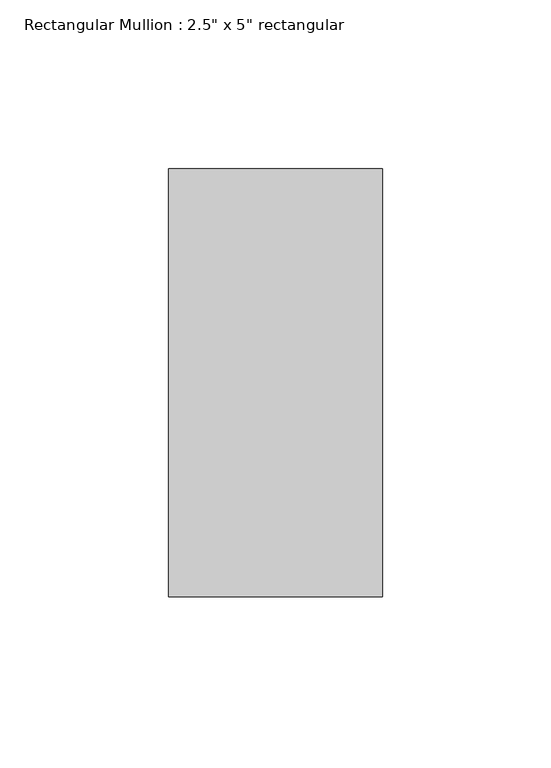
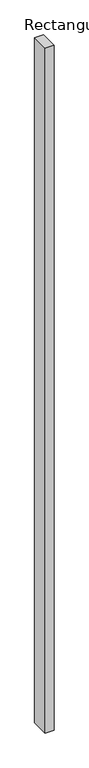
"""IFC4 building model written with IfcOpenShell, lengths in millimetres: member geometry."""

from ifc_helpers import new_model, si_unit, frame, origin, place, context, project, spatial, polyline, outline, extrude, source, transform, mapped, element, save


def member_7da84c5f(model_context):
    return source(origin(), model_context, "Body", "SweptSolid", [
        extrude(outline(polyline([(0.0, 63.5), (0.0, -63.5), (-63.5, -63.5), (-63.5, 63.5), (0.0, 63.5)])), frame((0.0, 0.0, -5078.5981466), z_axis=(0.0, 0.0, 1.0), x_axis=(1.0, 0.0, 0.0)), (0.0, 0.0, 1.0), 5078.5981466),
    ])


if __name__ == "__main__":
    model = new_model("IFC4")
    model_context = context("Model", 3, world=origin())
    ifc_project = project(units=[si_unit("LENGTHUNIT", "METRE", prefix="MILLI")], contexts=[model_context])
    site = spatial("IfcSite", under=ifc_project)
    building = spatial("IfcBuilding", under=site)
    placement = place(None, origin())
    member_shape = member_7da84c5f(model_context)
    element("IfcMember", 1, ObjectType="Rectangular Mullion : 2.5\" x 5\" rectangular", at=placement, inside=building, context=model_context, shape_type="MappedRepresentation", body=[
        mapped(member_shape, transform((0.0, 0.0, 0.0), x_axis=(1.0, 0.0, 0.0), y_axis=(0.0, 1.0, 0.0), z_axis=(0.0, 0.0, 1.0))),
    ])
    save(model, "model.ifc")

# Revit data of these elements
# Type "Rectangular Mullion : 2.5\" x 5\" rectangular"
#   built-in parameter 1007304 = 0.416667 (stored number, unit not read)
#   built-in parameter 1007301 = 0.104167 (stored number, unit not read)
#   built-in parameter 1007300 = 0.104167 (stored number, unit not read)
# Element 1 (IfcMember, "Rectangular Mullion : 2.5\" x 5\" rectangular")
#   Materials on its faces: "Aluminum"
# Materials
#   "Aluminum": class "Metal", colour RGB 247 247 247, transparency 0, Description = "Aluminum 6061", Cost = 0
